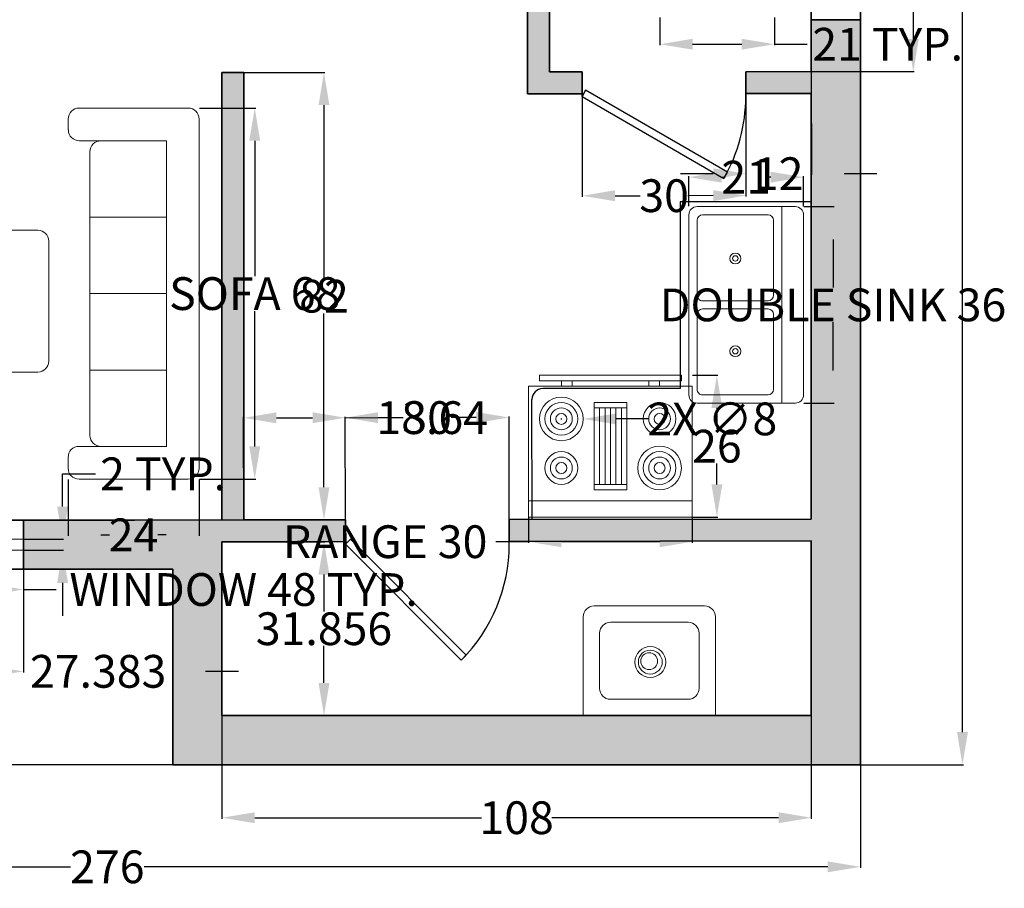
# Model space of a CAD drawing. Units: inches. Extents: x 98 to 487, y -240 to 141.
# Tile 2 of 5: x 251 to 431, y -240 to -81. Entities that reach past the tile are written whole.
import ezdxf

# ---------------------------------------------------------------- set-up
doc = ezdxf.new("R2010")
doc.units = ezdxf.units.IN
doc.header["$MEASUREMENT"] = 0
for name, color, linetype, lineweight in [('A-ANNO-DIMS', 2, 'Continuous', 18), ('A-DOOR', 3, 'Continuous', 25), ('A-EQPM', 9, 'Continuous', 18), ('A-FLOR-CASE', 8, 'Continuous', 25), ('A-FLOR-FIXT', 9, 'Continuous', 18), ('A-FURN', 8, 'Continuous', 18), ('A-GLAZ', 4, 'Continuous', 18), ('A-WALL', 7, 'Continuous', 35)]:
    doc.layers.add(name, color=color, linetype=linetype, lineweight=lineweight)
doc.layers.add('A-WALL-PATT', color=251, linetype='Continuous', lineweight=13, true_color=0x636466)
doc.styles.get("Standard").update_dxf_attribs({"font": 'arial.ttf'})
doc.dimstyles.get("Standard").update_dxf_attribs({"dimtxt": 6, "dimasz": 6, "dimexe": 0.18, "dimexo": 0.0625, "dimgap": 0.09, "dimtad": 0, "dimtih": 1, "dimtoh": 1, "dimdec": 0, "dimzin": 0, "dimdsep": 46, "dimlunit": 4, "dimtxsty": 'Standard', "dimcen": 0.09, "dimadec": 0, "dimazin": 0, "dimtfac": 1, "dimtdec": 0, "dimtofl": 0, "dimtmove": 0, "dimatfit": 3, "dimfxl": 1, "dimtolj": 1, "dimtzin": 0, "dimarcsym": 0})

# ---------------------------------------------------------------- blocks, each defined once
blk = doc.blocks.new('SOFA')
for p, q in [((-21.98, 0), (-2, 0)), ((-23.96, -4.02), (-23.98, -2.02)), ((0, -2), (0, -62)), ((-6, -6), (-21.96, -6)), ((-6, -62), (-6, -6)), ((-22, -62), (-6, -62)), ((0, -62), (0, -66)), ((-24, -66), (-24, -64)), ((-2, -68), (-22, -68))]:
    blk.add_line(p, q)
for points in [[(-6, -6), (-18, -6, 0.414214), (-20, -8), (-20, -20), (-6, -20)], [(-6, -48), (-20, -48), (-20, -60, 0.414214), (-18, -62), (-6, -62)]]:
    blk.add_lwpolyline(points, format="xyb", close=True)
for points in [[(-6, -20), (-20, -20), (-20, -34), (-6, -34)], [(-6, -34), (-20, -34), (-20, -48), (-6, -48)]]:
    blk.add_lwpolyline(points, close=True)
for centre, start, end in [((-21.98, -2), 90, 180.5593), ((-2, -2), 0, 90), ((-21.96, -4), 180.5593, 270), ((-22, -64), 90, 180), ((-22, -66), 180, 270), ((-2, -66), 270, 360)]:
    blk.add_arc(centre, 2, start, end)
blk = doc.blocks.new('*U12')
for p, q in [((0, 0), (0, 6)), ((40, 0), (40, 6))]:
    blk.add_line(p, q)
blk.add_lwpolyline([(0, 0), (28.28, -28.28), (29.52, -27.05), (1.24, 1.24)], close=True)
blk.add_arc((0, 0), 40, 315, 0)
blk = doc.blocks.new('*U9')
for p, q in [((0, 0), (0, 6)), ((40, 0), (40, 6))]:
    blk.add_line(p, q)
blk.add_lwpolyline([(0, 0), (34.64, -20), (35.52, -18.48), (0.87, 1.52)], close=True)
blk.add_arc((0, 0), 40, 330, 0)
blk = doc.blocks.new('Range-Oven - 30 in top')
for p, q in [((0, -3), (30, -3)), ((12, -6), (18, -6)), ((13, -20), (13, -6)), ((14, -6), (14, -20)), ((15, -20), (15, -6)), ((16, -6), (16, -20)), ((17, -20), (17, -6)), ((18, -20), (12, -20)), ((6, -24), (6, -25)), ((8, -25), (8, -24)), ((22, -25), (22, -24)), ((24, -24), (24, -25))]:
    blk.add_line(p, q)
for points in [[(0, -24), (0, 0), (30, 0), (30, -24)], [(12, -21), (12, -5), (18, -5), (18, -21)], [(2, -26), (2, -25), (28, -25), (28, -26)]]:
    blk.add_lwpolyline(points, close=True)
for centre, radius in [((6, -9), 4), ((6, -9), 3), ((6, -9), 2), ((24, -9), 3), ((24, -9), 2), ((6, -9), 1), ((24, -9), 1), ((24, -18), 4), ((6, -18), 3), ((6, -18), 2), ((24, -18), 3), ((24, -18), 2), ((6, -18), 1), ((24, -18), 1)]:
    blk.add_circle(centre, radius)
blk = doc.blocks.new('Sink-double - 36 in top')
for p, q in [((-18, -4), (18, -4)), ((-0.75, -18.5), (-0.75, -6.5)), ((0.75, -6.5), (0.75, -18.5))]:
    blk.add_line(p, q)
for points in [[(-16.5, 0), (16.5, 0)], [(-18, -19.5), (-18, -1.5)], [(18, -1.5), (18, -19.5)], [(-16.5, -18.5), (-16.5, -6.5)], [(-15.5, -5.5), (-1.75, -5.5)], [(1.75, -5.5), (15.5, -5.5)], [(16.5, -6.5), (16.5, -18.5)], [(-1.75, -19.5), (-15.5, -19.5)], [(15.5, -19.5), (1.75, -19.5)], [(16.5, -21), (-16.5, -21)]]:
    blk.add_lwpolyline(points)
for centre, radius in [((-8.5, -12.5), 1), ((-8.5, -12.5), 0.5), ((8.5, -12.5), 1), ((8.5, -12.5), 0.5)]:
    blk.add_circle(centre, radius)
for centre, radius, start, end in [((-16.5, -1.5), 1.5, 90, 180), ((16.5, -1.5), 1.5, 0, 90), ((-15.5, -6.5), 1, 90, 180), ((-1.75, -6.5), 1, 0, 90), ((1.75, -6.5), 1, 90, 180), ((15.5, -6.5), 1, 0, 90), ((-16.5, -19.5), 1.5, 180, 270), ((-15.5, -18.5), 1, 180, 270), ((-1.75, -18.5), 1, 270, 0), ((1.75, -18.5), 1, 180, 270), ((15.5, -18.5), 1, 270, 0), ((16.5, -19.5), 1.5, 270, 0)]:
    blk.add_arc(centre, radius, start, end)
blk = doc.blocks.new('GLAZ-48IN')
for p, q in [((48, 2), (0, 2)), ((48, 0), (0, 0))]:
    blk.add_line(p, q)
blk = doc.blocks.new('*D28')
at = {"layer": 'A-ANNO-DIMS', "color": 0, "lineweight": -2, "transparency": 16777216}
for p, q in [((203.38, -178.13), (203.38, -185.45)), ((251.38, -178.13), (251.38, -185.45)), ((209.38, -185.27), (245.38, -185.27)), ((251.38, -185.27), (257.38, -185.27))]:
    blk.add_line(p, q, dxfattribs=at)
at = {"layer": 'A-ANNO-DIMS', "color": 0, "transparency": 16777216}
for points in [[(209.38, -184.27), (209.38, -186.27), (203.38, -185.27)], [(245.38, -184.27), (245.38, -186.27), (251.38, -185.27)]]:
    blk.add_solid(points, dxfattribs=at)
at = {"layer": 'Defpoints', "color": 0, "transparency": 16777216}
for p in [(203.38, -178.07), (251.38, -178.07), (251.38, -185.27)]:
    blk.add_point(p, dxfattribs=at)
at = {"layer": 'A-ANNO-DIMS', "color": 0, "transparency": 16777216, "insert": (291.75, -185.27), "char_height": 6, "attachment_point": 5}
blk.add_mtext('\\A1;WINDOW 48 TYP.', dxfattribs=at)
blk = doc.blocks.new('*D29')
at = {"layer": 'A-ANNO-DIMS', "color": 0, "lineweight": -2, "transparency": 16777216}
for p, q in [((258.58, -170.07), (258.58, -164.07)), ((258.58, -164.07), (264.58, -164.07)), ((251.45, -176.07), (258.76, -176.07)), ((251.45, -178.07), (258.76, -178.07)), ((258.58, -184.07), (258.58, -190.07))]:
    blk.add_line(p, q, dxfattribs=at)
at = {"layer": 'A-ANNO-DIMS', "color": 0, "transparency": 16777216}
for points in [[(257.58, -170.07), (259.58, -170.07), (258.58, -176.07)], [(257.58, -184.07), (259.58, -184.07), (258.58, -178.07)]]:
    blk.add_solid(points, dxfattribs=at)
at = {"layer": 'Defpoints', "color": 0, "transparency": 16777216}
for p in [(251.38, -176.07), (258.58, -176.07), (251.38, -178.07)]:
    blk.add_point(p, dxfattribs=at)
at = {"layer": 'A-ANNO-DIMS', "color": 0, "transparency": 16777216, "insert": (277, -164.07), "char_height": 6, "attachment_point": 5}
blk.add_mtext('\\A1;2 TYP.', dxfattribs=at)
blk = doc.blocks.new('*D37')
at = {"layer": 'A-ANNO-DIMS', "color": 0, "lineweight": -2, "transparency": 16777216}
for p, q in [((368.02, -80.47), (368.02, -85.54)), ((389.02, -80.47), (389.02, -85.54)), ((374.02, -85.36), (383.02, -85.36)), ((389.02, -85.36), (395.02, -85.36))]:
    blk.add_line(p, q, dxfattribs=at)
at = {"layer": 'A-ANNO-DIMS', "color": 0, "transparency": 16777216}
for points in [[(374.02, -84.36), (374.02, -86.36), (368.02, -85.36)], [(383.02, -84.36), (383.02, -86.36), (389.02, -85.36)]]:
    blk.add_solid(points, dxfattribs=at)
at = {"layer": 'Defpoints', "color": 0, "transparency": 16777216}
for p in [(368.02, -80.4), (389.02, -80.4), (389.02, -85.36)]:
    blk.add_point(p, dxfattribs=at)
at = {"layer": 'A-ANNO-DIMS', "color": 0, "transparency": 16777216, "insert": (409.76, -85.36), "char_height": 6, "attachment_point": 5}
blk.add_mtext('\\A1;21 TYP.', dxfattribs=at)
blk = doc.blocks.new('*D40')
at = {"layer": 'A-ANNO-DIMS', "color": 0, "lineweight": -2, "transparency": 16777216}
for p, q in [((283.65, -97.05), (293.96, -97.05)), ((293.78, -103.05), (293.78, -127.86)), ((293.78, -159.05), (293.78, -134.25)), ((283.65, -165.05), (293.96, -165.05))]:
    blk.add_line(p, q, dxfattribs=at)
at = {"layer": 'A-ANNO-DIMS', "color": 0, "transparency": 16777216}
for points in [[(292.78, -103.05), (294.78, -103.05), (293.78, -97.05)], [(292.78, -159.05), (294.78, -159.05), (293.78, -165.05)]]:
    blk.add_solid(points, dxfattribs=at)
at = {"layer": 'Defpoints', "color": 0, "transparency": 16777216}
for p in [(283.58, -97.05), (293.78, -97.05), (283.58, -165.05)]:
    blk.add_point(p, dxfattribs=at)
at = {"layer": 'A-ANNO-DIMS', "color": 0, "transparency": 16777216, "insert": (293.78, -131.05), "char_height": 6, "attachment_point": 5}
blk.add_mtext('\\A1;SOFA 68', dxfattribs=at)
blk = doc.blocks.new('*D41')
at = {"layer": 'A-ANNO-DIMS', "color": 0, "lineweight": -2, "transparency": 16777216}
for p, q in [((259.58, -165.12), (259.58, -175.43)), ((283.58, -165.12), (283.58, -175.43)), ((265.58, -175.25), (267.16, -175.25)), ((277.58, -175.25), (276.01, -175.25))]:
    blk.add_line(p, q, dxfattribs=at)
at = {"layer": 'A-ANNO-DIMS', "color": 0, "transparency": 16777216}
for points in [[(265.58, -174.25), (265.58, -176.25), (259.58, -175.25)], [(277.58, -174.25), (277.58, -176.25), (283.58, -175.25)]]:
    blk.add_solid(points, dxfattribs=at)
at = {"layer": 'Defpoints', "color": 0, "transparency": 16777216}
for p in [(259.58, -165.05), (283.58, -165.05), (283.58, -175.25)]:
    blk.add_point(p, dxfattribs=at)
at = {"layer": 'A-ANNO-DIMS', "color": 0, "transparency": 16777216, "insert": (271.58, -175.25), "char_height": 6, "attachment_point": 5}
blk.add_mtext('\\A1;24', dxfattribs=at)
blk = doc.blocks.new('*D42')
at = {"layer": 'A-ANNO-DIMS', "color": 0, "lineweight": -2, "transparency": 16777216}
for p, q in [((343.97, -172.07), (343.97, -176.69)), ((373.97, -172.07), (373.97, -176.69)), ((343.97, -176.51), (337.97, -176.51)), ((367.97, -176.51), (349.97, -176.51))]:
    blk.add_line(p, q, dxfattribs=at)
at = {"layer": 'A-ANNO-DIMS', "color": 0, "transparency": 16777216}
for points in [[(349.97, -175.51), (349.97, -177.51), (343.97, -176.51)], [(367.97, -175.51), (367.97, -177.51), (373.97, -176.51)]]:
    blk.add_solid(points, dxfattribs=at)
at = {"layer": 'Defpoints', "color": 0, "transparency": 16777216}
for p in [(343.97, -172.01), (373.97, -172.01), (343.97, -176.51)]:
    blk.add_point(p, dxfattribs=at)
at = {"layer": 'A-ANNO-DIMS', "color": 0, "transparency": 16777216, "insert": (317.68, -176.51), "char_height": 6, "attachment_point": 5}
blk.add_mtext('\\A1;RANGE 30', dxfattribs=at)
blk = doc.blocks.new('*D43')
at = {"layer": 'A-ANNO-DIMS', "color": 0, "lineweight": -2, "transparency": 16777216}
for p, q in [((374.03, -146.01), (378.65, -146.01)), ((378.47, -152.01), (378.47, -155.85)), ((378.47, -166.01), (378.47, -162.16)), ((374.03, -172.01), (378.65, -172.01))]:
    blk.add_line(p, q, dxfattribs=at)
at = {"layer": 'A-ANNO-DIMS', "color": 0, "transparency": 16777216}
for points in [[(377.47, -152.01), (379.47, -152.01), (378.47, -146.01)], [(377.47, -166.01), (379.47, -166.01), (378.47, -172.01)]]:
    blk.add_solid(points, dxfattribs=at)
at = {"layer": 'Defpoints', "color": 0, "transparency": 16777216}
for p in [(373.97, -146.01), (373.97, -172.01), (378.47, -172.01)]:
    blk.add_point(p, dxfattribs=at)
at = {"layer": 'A-ANNO-DIMS', "color": 0, "transparency": 16777216, "insert": (378.47, -159.01), "char_height": 6, "attachment_point": 5}
blk.add_mtext('\\A1;26', dxfattribs=at)
blk = doc.blocks.new('*D44')
at = {"layer": 'A-ANNO-DIMS', "color": 0, "lineweight": -2, "transparency": 16777216}
for p, q in [((394.41, -115.12), (399.93, -115.12)), ((399.75, -121.12), (399.75, -129.92)), ((399.75, -145.12), (399.75, -136.31)), ((394.41, -151.12), (399.93, -151.12))]:
    blk.add_line(p, q, dxfattribs=at)
at = {"layer": 'A-ANNO-DIMS', "color": 0, "transparency": 16777216}
for points in [[(398.75, -121.12), (400.75, -121.12), (399.75, -115.12)], [(398.75, -145.12), (400.75, -145.12), (399.75, -151.12)]]:
    blk.add_solid(points, dxfattribs=at)
at = {"layer": 'Defpoints', "color": 0, "transparency": 16777216}
for p in [(394.35, -115.12), (394.35, -151.12), (399.75, -151.12)]:
    blk.add_point(p, dxfattribs=at)
at = {"layer": 'A-ANNO-DIMS', "color": 0, "transparency": 16777216, "insert": (399.75, -133.12), "char_height": 6, "attachment_point": 5}
blk.add_mtext('\\A1;DOUBLE SINK 36', dxfattribs=at)
blk = doc.blocks.new('*D45')
at = {"layer": 'A-ANNO-DIMS', "color": 0, "lineweight": -2, "transparency": 16777216}
for p, q in [((373.35, -115.05), (373.35, -109.54)), ((379.35, -109.72), (379.99, -109.72)), ((388.35, -109.72), (387.71, -109.72)), ((394.35, -115.05), (394.35, -109.54))]:
    blk.add_line(p, q, dxfattribs=at)
at = {"layer": 'A-ANNO-DIMS', "color": 0, "transparency": 16777216}
for points in [[(379.35, -108.72), (379.35, -110.72), (373.35, -109.72)], [(388.35, -108.72), (388.35, -110.72), (394.35, -109.72)]]:
    blk.add_solid(points, dxfattribs=at)
at = {"layer": 'Defpoints', "color": 0, "transparency": 16777216}
for p in [(394.35, -109.72), (373.35, -115.12), (394.35, -115.12)]:
    blk.add_point(p, dxfattribs=at)
at = {"layer": 'A-ANNO-DIMS', "color": 0, "transparency": 16777216, "insert": (383.85, -109.72), "char_height": 6, "attachment_point": 5}
blk.add_mtext('\\A1;21', dxfattribs=at)
blk = doc.blocks.new('*D46')
at = {"layer": 'A-ANNO-DIMS', "color": 0, "lineweight": -2, "transparency": 16777216}
for p, q in [((128.77, -181.8), (128.77, -236.26)), ((404.77, -217.44), (404.77, -236.26)), ((134.77, -236.08), (260, -236.08)), ((398.77, -236.08), (273.53, -236.08))]:
    blk.add_line(p, q, dxfattribs=at)
at = {"layer": 'A-ANNO-DIMS', "color": 0, "transparency": 16777216}
for points in [[(134.77, -235.08), (134.77, -237.08), (128.77, -236.08)], [(398.77, -235.08), (398.77, -237.08), (404.77, -236.08)]]:
    blk.add_solid(points, dxfattribs=at)
at = {"layer": 'Defpoints', "color": 0, "transparency": 16777216}
for p in [(128.77, -181.73), (404.77, -217.38), (404.77, -236.08)]:
    blk.add_point(p, dxfattribs=at)
at = {"layer": 'A-ANNO-DIMS', "color": 0, "transparency": 16777216, "insert": (266.77, -236.08), "char_height": 6, "attachment_point": 5}
blk.add_mtext('\\A1;276', dxfattribs=at)
blk = doc.blocks.new('*D47')
at = {"layer": 'A-ANNO-DIMS', "color": 0, "lineweight": -2, "transparency": 16777216}
for p, q in [((404.83, 118.64), (423.65, 118.64)), ((423.47, 112.64), (423.47, -46.22)), ((423.47, -211.38), (423.47, -52.53)), ((404.83, -217.38), (423.65, -217.38))]:
    blk.add_line(p, q, dxfattribs=at)
at = {"layer": 'A-ANNO-DIMS', "color": 0, "transparency": 16777216}
for points in [[(422.47, 112.64), (424.47, 112.64), (423.47, 118.64)], [(422.47, -211.38), (424.47, -211.38), (423.47, -217.38)]]:
    blk.add_solid(points, dxfattribs=at)
at = {"layer": 'Defpoints', "color": 0, "transparency": 16777216}
for p in [(404.77, 118.64), (404.77, -217.38), (423.47, -217.38)]:
    blk.add_point(p, dxfattribs=at)
at = {"layer": 'A-ANNO-DIMS', "color": 0, "transparency": 16777216, "insert": (423.47, -49.37), "char_height": 6, "attachment_point": 5}
blk.add_mtext('\\A1;336', dxfattribs=at)
blk = doc.blocks.new('*D58')
at = {"layer": 'A-ANNO-DIMS', "color": 0, "lineweight": -2, "transparency": 16777216}
for p, q in [((278.7, -181.55), (109.89, -181.55)), ((110.07, -187.55), (110.07, -196.31)), ((110.07, -211.38), (110.07, -202.62)), ((278.7, -217.38), (109.89, -217.38))]:
    blk.add_line(p, q, dxfattribs=at)
at = {"layer": 'A-ANNO-DIMS', "color": 0, "transparency": 16777216}
for points in [[(109.07, -187.55), (111.07, -187.55), (110.07, -181.55)], [(109.07, -211.38), (111.07, -211.38), (110.07, -217.38)]]:
    blk.add_solid(points, dxfattribs=at)
at = {"layer": 'Defpoints', "color": 0, "transparency": 16777216}
for p in [(278.77, -181.55), (110.07, -217.38), (278.77, -217.38)]:
    blk.add_point(p, dxfattribs=at)
at = {"layer": 'A-ANNO-DIMS', "color": 0, "transparency": 16777216, "insert": (110.07, -199.46), "char_height": 6, "attachment_point": 5}
blk.add_mtext('\\A1;35.83', dxfattribs=at)
blk = doc.blocks.new('*D62')
at = {"layer": 'A-ANNO-DIMS', "color": 0, "lineweight": -2, "transparency": 16777216}
for p, q in [((251.38, -181.63), (251.4, -200.45)), ((278.77, -181.61), (278.78, -200.43)), ((245.4, -200.27), (239.4, -200.28)), ((284.78, -200.24), (290.78, -200.24))]:
    blk.add_line(p, q, dxfattribs=at)
at = {"layer": 'A-ANNO-DIMS', "color": 0, "transparency": 16777216}
for points in [[(245.4, -199.27), (245.4, -201.27), (251.4, -200.27)], [(284.78, -199.24), (284.78, -201.24), (278.78, -200.25)]]:
    blk.add_solid(points, dxfattribs=at)
at = {"layer": 'Defpoints', "color": 0, "transparency": 16777216}
for p in [(251.38, -181.57), (278.77, -181.55), (251.4, -200.27)]:
    blk.add_point(p, dxfattribs=at)
at = {"layer": 'A-ANNO-DIMS', "color": 0, "transparency": 16777216, "insert": (265.09, -200.26), "char_height": 6, "attachment_point": 5}
blk.add_mtext('\\A1;27.383', dxfattribs=at)
blk = doc.blocks.new('*D63')
at = {"layer": 'A-ANNO-DIMS', "color": 0, "lineweight": -2, "transparency": 16777216}
for p, q in [((287.77, -208.44), (287.77, -227.26)), ((395.77, -208.44), (395.77, -227.26)), ((293.77, -227.08), (335.32, -227.08)), ((389.77, -227.08), (348.21, -227.08))]:
    blk.add_line(p, q, dxfattribs=at)
at = {"layer": 'A-ANNO-DIMS', "color": 0, "transparency": 16777216}
for points in [[(293.77, -226.08), (293.77, -228.08), (287.77, -227.08)], [(389.77, -226.08), (389.77, -228.08), (395.77, -227.08)]]:
    blk.add_solid(points, dxfattribs=at)
at = {"layer": 'Defpoints', "color": 0, "transparency": 16777216}
for p in [(287.77, -208.38), (395.77, -208.38), (287.77, -227.08)]:
    blk.add_point(p, dxfattribs=at)
at = {"layer": 'A-ANNO-DIMS', "color": 0, "transparency": 16777216, "insert": (341.77, -227.08), "char_height": 6, "attachment_point": 5}
blk.add_mtext('\\A1;108', dxfattribs=at)
blk = doc.blocks.new('*D64')
at = {"layer": 'A-ANNO-DIMS', "color": 0, "lineweight": -2, "transparency": 16777216}
for p, q in [((287.83, -176.52), (306.65, -176.52)), ((306.47, -182.52), (306.47, -189.29)), ((306.47, -202.38), (306.47, -195.6)), ((287.83, -208.38), (306.65, -208.38))]:
    blk.add_line(p, q, dxfattribs=at)
at = {"layer": 'A-ANNO-DIMS', "color": 0, "transparency": 16777216}
for points in [[(305.47, -182.52), (307.47, -182.52), (306.47, -176.52)], [(305.47, -202.38), (307.47, -202.38), (306.47, -208.38)]]:
    blk.add_solid(points, dxfattribs=at)
at = {"layer": 'Defpoints', "color": 0, "transparency": 16777216}
for p in [(287.77, -176.52), (287.77, -208.38), (306.47, -208.38)]:
    blk.add_point(p, dxfattribs=at)
at = {"layer": 'A-ANNO-DIMS', "color": 0, "transparency": 16777216, "insert": (306.47, -192.45), "char_height": 6, "attachment_point": 5}
blk.add_mtext('\\A1;31.856', dxfattribs=at)
blk = doc.blocks.new('*D66')
at = {"layer": 'A-ANNO-DIMS', "color": 0, "lineweight": -2, "transparency": 16777216}
for p, q in [((395.83, -42.38), (414.65, -42.38)), ((414.47, -48.38), (414.47, -63.22)), ((414.47, -84.38), (414.47, -69.53)), ((395.83, -90.38), (414.65, -90.38))]:
    blk.add_line(p, q, dxfattribs=at)
at = {"layer": 'A-ANNO-DIMS', "color": 0, "transparency": 16777216}
for points in [[(413.47, -48.38), (415.47, -48.38), (414.47, -42.38)], [(413.47, -84.38), (415.47, -84.38), (414.47, -90.38)]]:
    blk.add_solid(points, dxfattribs=at)
at = {"layer": 'Defpoints', "color": 0, "transparency": 16777216}
for p in [(395.77, -42.38), (395.77, -90.38), (414.47, -90.38)]:
    blk.add_point(p, dxfattribs=at)
at = {"layer": 'A-ANNO-DIMS', "color": 0, "transparency": 16777216, "insert": (414.47, -66.38), "char_height": 6, "attachment_point": 5}
blk.add_mtext('\\A1;48', dxfattribs=at)
blk = doc.blocks.new('*D68')
at = {"layer": 'A-ANNO-DIMS', "color": 0, "lineweight": -2, "transparency": 16777216}
for p, q in [((353.77, -94.5), (353.8, -113.31)), ((383.77, -94.46), (383.8, -113.27)), ((359.8, -113.12), (364.42, -113.12)), ((377.8, -113.1), (373.17, -113.11))]:
    blk.add_line(p, q, dxfattribs=at)
at = {"layer": 'A-ANNO-DIMS', "color": 0, "transparency": 16777216}
for points in [[(359.8, -112.12), (359.8, -114.12), (353.8, -113.13)], [(377.8, -112.1), (377.8, -114.1), (383.8, -113.09)]]:
    blk.add_solid(points, dxfattribs=at)
at = {"layer": 'Defpoints', "color": 0, "transparency": 16777216}
for p in [(353.77, -94.43), (383.77, -94.39), (353.8, -113.13)]:
    blk.add_point(p, dxfattribs=at)
at = {"layer": 'A-ANNO-DIMS', "color": 0, "transparency": 16777216, "insert": (368.8, -113.11), "char_height": 6, "attachment_point": 5}
blk.add_mtext('\\A1;30', dxfattribs=at)
blk = doc.blocks.new('*D69')
at = {"layer": 'A-ANNO-DIMS', "color": 0, "lineweight": -2, "transparency": 16777216}
for p, q in [((383.77, -90.46), (383.79, -109.27)), ((395.77, -90.44), (395.79, -109.26)), ((377.79, -109.1), (371.79, -109.11)), ((401.79, -109.07), (407.79, -109.06))]:
    blk.add_line(p, q, dxfattribs=at)
at = {"layer": 'A-ANNO-DIMS', "color": 0, "transparency": 16777216}
for points in [[(377.79, -108.1), (377.79, -110.1), (383.79, -109.09)], [(401.79, -108.07), (401.79, -110.07), (395.79, -109.08)]]:
    blk.add_solid(points, dxfattribs=at)
at = {"layer": 'Defpoints', "color": 0, "transparency": 16777216}
for p in [(383.77, -90.39), (395.77, -90.38), (383.79, -109.09)]:
    blk.add_point(p, dxfattribs=at)
at = {"layer": 'A-ANNO-DIMS', "color": 0, "transparency": 16777216, "insert": (389.79, -109.08), "char_height": 6, "attachment_point": 5}
blk.add_mtext('\\A1;12', dxfattribs=at)
blk = doc.blocks.new('*D79')
at = {"layer": 'A-ANNO-DIMS', "color": 0, "lineweight": -2, "transparency": 16777216}
for p, q in [((291.77, -172.45), (291.74, -153.64)), ((297.74, -153.81), (304.38, -153.8)), ((310.41, -172.43), (310.38, -153.61)), ((310.38, -153.79), (316.38, -153.78))]:
    blk.add_line(p, q, dxfattribs=at)
at = {"layer": 'A-ANNO-DIMS', "color": 0, "transparency": 16777216}
for points in [[(297.74, -152.81), (297.74, -154.81), (291.74, -153.82)], [(304.38, -152.8), (304.38, -154.8), (310.38, -153.79)]]:
    blk.add_solid(points, dxfattribs=at)
at = {"layer": 'Defpoints', "color": 0, "transparency": 16777216}
for p in [(310.38, -153.79), (291.77, -172.52), (310.41, -172.49)]:
    blk.add_point(p, dxfattribs=at)
at = {"layer": 'A-ANNO-DIMS', "color": 0, "transparency": 16777216, "insert": (326.3, -153.78), "char_height": 6, "attachment_point": 5}
blk.add_mtext('\\A1;18.64', dxfattribs=at)
blk = doc.blocks.new('*D80')
at = {"layer": 'A-ANNO-DIMS', "color": 0, "lineweight": -2, "transparency": 16777216}
for p, q in [((310.41, -172.43), (310.38, -153.61)), ((316.38, -153.78), (321.01, -153.78)), ((334.38, -153.76), (329.76, -153.76)), ((340.41, -172.39), (340.38, -153.57))]:
    blk.add_line(p, q, dxfattribs=at)
at = {"layer": 'A-ANNO-DIMS', "color": 0, "transparency": 16777216}
for points in [[(316.38, -152.78), (316.38, -154.78), (310.38, -153.79)], [(334.38, -152.76), (334.38, -154.76), (340.38, -153.75)]]:
    blk.add_solid(points, dxfattribs=at)
at = {"layer": 'Defpoints', "color": 0, "transparency": 16777216}
for p in [(340.38, -153.75), (310.41, -172.49), (340.41, -172.45)]:
    blk.add_point(p, dxfattribs=at)
at = {"layer": 'A-ANNO-DIMS', "color": 0, "transparency": 16777216, "insert": (325.38, -153.77), "char_height": 6, "attachment_point": 5}
blk.add_mtext('\\A1;30', dxfattribs=at)
blk = doc.blocks.new('*D81')
at = {"layer": 'A-ANNO-DIMS', "color": 0, "lineweight": -2, "transparency": 16777216}
for p, q in [((287.83, -90.52), (306.65, -90.52)), ((306.47, -96.52), (306.47, -128.37)), ((306.47, -166.52), (306.47, -134.67)), ((287.83, -172.52), (306.65, -172.52))]:
    blk.add_line(p, q, dxfattribs=at)
at = {"layer": 'A-ANNO-DIMS', "color": 0, "transparency": 16777216}
for points in [[(305.47, -96.52), (307.47, -96.52), (306.47, -90.52)], [(305.47, -166.52), (307.47, -166.52), (306.47, -172.52)]]:
    blk.add_solid(points, dxfattribs=at)
at = {"layer": 'Defpoints', "color": 0, "transparency": 16777216}
for p in [(287.77, -90.52), (287.77, -172.52), (306.47, -172.52)]:
    blk.add_point(p, dxfattribs=at)
at = {"layer": 'A-ANNO-DIMS', "color": 0, "transparency": 16777216, "insert": (306.47, -131.52), "char_height": 6, "attachment_point": 5}
blk.add_mtext('\\A1;82', dxfattribs=at)
blk = doc.blocks.new('*D87')
at = {"layer": 'A-ANNO-DIMS', "color": 0, "lineweight": -2, "transparency": 16777216}
for p, q in [((349.88, -154.01), (350.06, -154.01)), ((349.97, -154.1), (349.97, -153.92)), ((365.97, -154.01), (359.97, -154.01))]:
    blk.add_line(p, q, dxfattribs=at)
at = {"layer": 'A-ANNO-DIMS', "color": 0, "transparency": 16777216}
blk.add_solid([(359.97, -153.01), (359.97, -155.01), (353.97, -154.01)], dxfattribs=at)
at = {"layer": 'Defpoints', "color": 0, "transparency": 16777216}
for p in [(345.97, -154.01), (353.97, -154.01)]:
    blk.add_point(p, dxfattribs=at)
at = {"layer": 'A-ANNO-DIMS', "color": 0, "transparency": 16777216, "insert": (377.63, -154.01), "char_height": 6, "attachment_point": 5}
blk.add_mtext('\\A1;2X ∅8', dxfattribs=at)

msp = doc.modelspace()

# ---------------------------------------------------------------- hatches: boundary and pattern name
at = {"layer": 'A-WALL-PATT'}
h = msp.add_hatch(color=256, dxfattribs=at)
h.dxf.hatch_style = 1
h.paths.add_polyline_path([(404.7663, -26.698), (395.7663, -26.698), (395.7663, -38.3769), (347.7663, -38.4409), (347.7583, -32.4409), (343.7663, -32.4462), (343.7663, -42.4462), (343.7663, -90.4463), (343.7716, -94.4463), (353.7716, -94.4329), (353.7663, -90.4329), (347.7663, -90.441), (347.7663, -42.4409), (395.7663, -42.3769), (395.7663, -56.8658), (404.7663, -56.8658)])
h = msp.add_hatch(color=256, dxfattribs=at)
h.dxf.hatch_style = 1
h.paths.add_polyline_path([(404.7663, -80.8658), (395.7663, -80.8658), (395.7663, -90.3769), (383.7716, -90.3929), (383.7716, -94.3929), (395.7663, -94.3769), (395.7663, -172.3767), (340.4126, -172.4506), (340.4126, -176.4506), (395.7663, -176.3767), (395.7663, -208.3767), (287.7663, -208.3767), (287.7663, -176.5208), (310.4126, -176.4906), (310.4073, -172.4906), (291.7663, -172.5155), (291.7663, -94.5157), (291.7663, -90.5157), (287.7663, -90.521), (287.7663, -172.5208), (271.7663, -172.5422), (251.3829, -172.5693), (251.3829, -181.5694), (266.7305, -181.5489), (278.7663, -181.5489), (278.7663, -208.3767), (278.7663, -217.3767), (395.7663, -217.3767), (404.7663, -217.3767), (404.7663, -172.3767)])

# ---------------------------------------------------------------- linework, layer by layer
at = {"layer": 'A-FLOR-CASE'}
for p, q in [((395.7663, -114.2297), (371.7663, -114.2297)), ((371.7663, -114.2297), (371.7663, -148.4087)), ((371.7663, -148.4087), (346.5788, -148.4423)), ((344.6108, -172.445), (344.5815, -150.445))]:
    msp.add_line(p, q, dxfattribs=at)
msp.add_arc((346.5814, -150.4423), 2, 90.07644, 180.07644, dxfattribs=at)
at = {"layer": 'A-FLOR-FIXT'}
for points in [[(378.2043, -208.3767), (353.9764, -208.3767), (353.9764, -190.257, -0.41421356), (355.9764, -188.257), (376.2043, -188.257, -0.41421356), (378.2043, -190.257)], [(373.2043, -205.3767), (358.9764, -205.3767, -0.41421356), (356.9764, -203.3767), (356.9764, -193.257, -0.41421356), (358.9764, -191.257), (373.2043, -191.257, -0.41421356), (375.2043, -193.257), (375.2043, -203.3767, -0.41421356)]]:
    msp.add_lwpolyline(points, format="xyb", close=True, dxfattribs=at)
for centre, radius in [((366.2699, -198.5632), 2.8329), ((366.2699, -198.5632), 2.1901), ((366.0687, -198.4021), 1.5437)]:
    msp.add_circle(centre, radius, dxfattribs=at)
at = {"layer": 'A-FURN'}
msp.add_lwpolyline([(254.0396, -119.4274), (232.0396, -119.4274, 0.41421356), (230.0396, -121.4274), (230.0396, -143.4274, 0.41421356), (232.0396, -145.4274), (254.0396, -145.4274, 0.41421356), (256.0396, -143.4274), (256.0396, -121.4274, 0.41421356)], format="xyb", close=True, dxfattribs=at)
at = {"layer": 'A-WALL'}
for p, q in [((343.7663, -42.3769), (343.7663, -90.4463)), ((347.7663, -42.3769), (347.7663, -90.441)), ((395.7663, -42.3769), (395.7663, -90.3769)), ((404.7663, -80.8658), (395.7663, -80.8658)), ((287.7663, -90.521), (291.7663, -90.5157)), ((287.7663, -90.521), (287.7663, -172.5208)), ((291.7663, -94.5157), (291.7663, -90.5157)), ((343.7663, -90.4463), (343.7716, -94.4463)), ((347.7663, -90.441), (353.7663, -90.4329)), ((353.7663, -90.4329), (353.7716, -94.4329)), ((383.7663, -90.3929), (395.7663, -90.3769)), ((383.7663, -90.3929), (383.7716, -94.3929)), ((291.7663, -94.5157), (291.7663, -172.5155)), ((343.7716, -94.4463), (353.7716, -94.4329)), ((383.7716, -94.3929), (395.7663, -94.3769)), ((395.7663, -94.3769), (395.7663, -172.3767)), ((271.7663, -172.5422), (173.7655, -172.6729)), ((251.3829, -172.5694), (251.3829, -181.5694)), ((287.7663, -172.5208), (271.7663, -172.5422)), ((310.4073, -172.4906), (291.7663, -172.5155)), ((310.4073, -172.4906), (310.4126, -176.4906)), ((395.7663, -172.3767), (340.4073, -172.4506)), ((340.4073, -172.4506), (340.4126, -176.4506)), ((404.7663, -172.3767), (404.7663, -217.3767)), ((310.4126, -176.4906), (287.7663, -176.5208)), ((287.7663, -176.5208), (287.7663, -208.3767)), ((395.7716, -176.3767), (340.4126, -176.4506)), ((395.7663, -176.3767), (395.7663, -208.3767)), ((266.7305, -181.5489), (278.7663, -181.5489)), ((278.7663, -181.5489), (278.7663, -208.3767)), ((278.7663, -208.3767), (278.7663, -217.3767)), ((395.7663, -208.3767), (287.7663, -208.3767)), ((395.7663, -217.3767), (278.7663, -217.3767)), ((395.7663, -217.3767), (404.7663, -217.3767))]:
    msp.add_line(p, q, dxfattribs=at)
for points in [[(143.7775, -181.7129), (128.7655, -181.7329), (128.7655, 118.2671), (404.7663, 118.6353), (404.7663, -181.3647)], [(266.7305, -181.5489), (173.7775, -181.6729)]]:
    msp.add_lwpolyline(points, dxfattribs=at)

# ---------------------------------------------------------------- block references
at = {"layer": 'A-DOOR', "xscale": 0.75, "yscale": 0.75, "zscale": 0.75}
for name, p in [('*U9', (353.7663, -94.9329)), ('*U12', (310.4133, -176.9906))]:
    msp.add_blockref(name, p, dxfattribs=at)
at = {"layer": 'A-EQPM', "rotation": 180}
msp.add_blockref('Range-Oven - 30 in top', (373.9687, -172.0061), dxfattribs=at)
at = {"layer": 'A-FLOR-FIXT', "rotation": 270}
msp.add_blockref('Sink-double - 36 in top', (394.3467, -133.1165), dxfattribs=at)
at = {"layer": 'A-FURN'}
msp.add_blockref('SOFA', (283.5845, -97.0529), dxfattribs=at)
at = {"layer": 'A-GLAZ'}
msp.add_blockref('GLAZ-48IN', (203.3825, -178.0689), dxfattribs=at)

# ---------------------------------------------------------------- dimensions: what is measured, and where the dimension line sits
at = {"layer": 'A-ANNO-DIMS'}
for base, p1, p2, angle, override, picture, middle in [((423.4663, -217.3767), (404.7663, 118.6353), (404.7663, -217.3767), 90, {"dimdec": 0, "dimlfac": 1, "dimrnd": 0, "dimzin": 0, "dimdsep": 46, "dimlunit": 2}, '*D47', (423.4663, -49.3707)), ((414.4663, -90.3769), (395.7663, -42.3769), (395.7663, -90.3769), 270, {"dimdec": 0, "dimlfac": 1, "dimrnd": 0, "dimzin": 0, "dimdsep": 46, "dimlunit": 2}, '*D66', (414.4663, -66.3769)), ((306.4663, -172.5208), (287.7663, -90.521), (287.7663, -172.5208), 270, {"dimdec": 0, "dimlfac": 1, "dimrnd": 0, "dimzin": 0, "dimdsep": 46, "dimlunit": 2}, '*D81', (306.4663, -131.5209)), ((383.7912, -109.0929), (395.7663, -90.3769), (383.7663, -90.3929), 180.07644, {"dimdec": 0, "dimlfac": 1, "dimrnd": 0, "dimzin": 0, "dimdsep": 46, "dimlunit": 2}, '*D69', (389.7912, -109.0849)), ((353.7966, -113.1329), (383.7716, -94.3929), (353.7716, -94.4329), 180.07644, {"dimdec": 0, "dimlfac": 1, "dimrnd": 0, "dimzin": 0, "dimdsep": 46, "dimlunit": 2}, '*D68', (368.7966, -113.1129)), ((378.4687, -172.0061), (373.9687, -146.0061), (373.9687, -172.0061), 270, {"dimdec": 0, "dimlfac": 1, "dimrnd": 0, "dimzin": 0, "dimdsep": 46, "dimlunit": 2}, '*D43', (378.4687, -159.0061)), ((310.3823, -153.7906), (291.7663, -172.5155), (310.4073, -172.4906), 0.07644, {"dimdec": 2, "dimlfac": 1, "dimrnd": 0, "dimzin": 0, "dimdsep": 46, "dimlunit": 2}, '*D79', (326.3011, -153.7826)), ((340.3823, -153.7506), (310.4073, -172.4906), (340.4073, -172.4506), 0.07644, {"dimdec": 0, "dimlfac": 1, "dimrnd": 0, "dimzin": 0, "dimdsep": 46, "dimlunit": 2}, '*D80', (325.3823, -153.7706)), ((306.4663, -208.3767), (287.7663, -176.5208), (287.7663, -208.3767), 270, {"dimdec": 3, "dimlfac": 1, "dimrnd": 0, "dimzin": 0, "dimdsep": 46, "dimlunit": 2}, '*D64', (306.4663, -192.4488)), ((110.0655, -217.3767), (278.7663, -181.5489), (278.7663, -217.3767), 90, {"dimdec": 2, "dimlfac": 1, "dimrnd": 0, "dimzin": 0, "dimdsep": 46, "dimlunit": 2}, '*D58', (110.0655, -199.4628)), ((251.3968, -200.2694), (278.7663, -181.5489), (251.3829, -181.5694), 180.042842, {"dimdec": 3, "dimlfac": 1, "dimrnd": 0, "dimzin": 0, "dimdsep": 46, "dimlunit": 2}, '*D62', (265.0886, -200.2591)), ((287.7663, -227.0767), (395.7663, -208.3767), (287.7663, -208.3767), 180, {"dimdec": 0, "dimlfac": 1, "dimrnd": 0, "dimzin": 0, "dimdsep": 46, "dimlunit": 2}, '*D63', (341.7663, -227.0767))]:
    dim = msp.add_linear_dim(base=base, p1=p1, p2=p2, angle=angle, dimstyle='Standard', override=override, dxfattribs=at)
    dim.commit()
    dim.dimension.update_dxf_attribs({"geometry": picture, "text_midpoint": middle})
for base, p1, p2, text, picture, middle in [((389.0194, -85.3611), (368.0194, -80.4041), (389.0194, -80.4041), '<> TYP.', '*D37', (409.7635, -85.3611)), ((251.3829, -185.2694), (203.3829, -178.0694), (251.3829, -178.0694), 'WINDOW <> TYP.', '*D28', (291.7519, -185.2694))]:
    dim = msp.add_linear_dim(base=base, p1=p1, p2=p2, text=text, dimstyle='Standard', override={"dimdec": 0, "dimlfac": 1, "dimrnd": 0, "dimzin": 0, "dimdsep": 46, "dimlunit": 2}, dxfattribs=at)
    dim.commit()
    dim.dimension.update_dxf_attribs({"geometry": picture, "text_midpoint": middle})
for base, p1, p2, angle, text, picture, middle in [((293.7845, -97.0529), (283.5845, -165.0529), (283.5845, -97.0529), 90, 'SOFA <>', '*D40', (293.7845, -131.0529)), ((399.7467, -151.1165), (394.3467, -115.1165), (394.3467, -151.1165), 270, 'DOUBLE SINK <>', '*D44', (399.7467, -133.1165)), ((258.5829, -176.0694), (251.3829, -178.0694), (251.3829, -176.0694), 90, '<> TYP.', '*D29', (276.9962, -164.0694)), ((343.9687, -176.5061), (373.9687, -172.0061), (343.9687, -172.0061), 180, 'RANGE <>', '*D42', (317.6788, -176.5061))]:
    dim = msp.add_linear_dim(base=base, p1=p1, p2=p2, angle=angle, text=text, dimstyle='Standard', override={"dimdec": 0, "dimlfac": 1, "dimrnd": 0, "dimzin": 0, "dimdsep": 46, "dimlunit": 2}, dxfattribs=at)
    dim.commit()
    dim.dimension.update_dxf_attribs({"geometry": picture, "text_midpoint": middle})
for base, p1, p2, picture, middle in [((394.3467, -109.7165), (373.3467, -115.1165), (394.3467, -115.1165), '*D45', (383.8467, -109.7165)), ((283.5845, -175.2529), (259.5845, -165.0529), (283.5845, -165.0529), '*D41', (271.5845, -175.2529)), ((404.7663, -236.0767), (128.7655, -181.7329), (404.7663, -217.3767), '*D46', (266.7659, -236.0767))]:
    dim = msp.add_linear_dim(base=base, p1=p1, p2=p2, dimstyle='Standard', override={"dimdec": 0, "dimlfac": 1, "dimrnd": 0, "dimzin": 0, "dimdsep": 46, "dimlunit": 2}, dxfattribs=at)
    dim.commit()
    dim.dimension.update_dxf_attribs({"geometry": picture, "text_midpoint": middle})
dim = msp.add_diameter_dim_2p(p1=(345.9687, -154.0062), p2=(353.9687, -154.006), text='2X <>', dimstyle='Standard', override={"dimdec": 0, "dimlfac": 1, "dimrnd": 0, "dimzin": 0, "dimdsep": 46, "dimlunit": 2}, dxfattribs=at)
dim.commit()
dim.dimension.update_dxf_attribs({"geometry": '*D87', "text_midpoint": (365.9687, -154.0057), "dimtype": 163})

doc.saveas('drawing.dxf')
